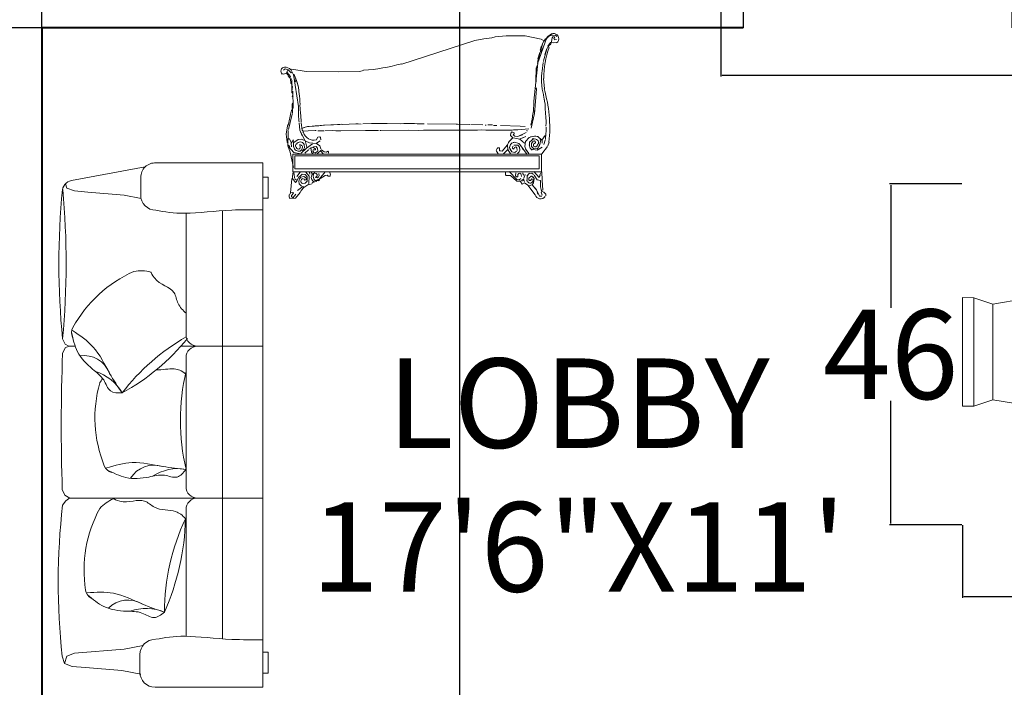
# Model space of a CAD drawing. Units: inches. Extents: x -124 to 612, y -69 to 524.
# Tile 4 of 9: x 16 to 148, y 240 to 329. Entities that reach past the tile are written whole.
import ezdxf
from ezdxf.enums import TextEntityAlignment as Align

# ---------------------------------------------------------------- set-up
doc = ezdxf.new("R2010")
doc.units = ezdxf.units.IN
doc.header["$MEASUREMENT"] = 0
for name, color, linetype, lineweight in [('A-ANNO-DIMS', 2, 'Continuous', 18), ('A-AREA-IDEN', 1, 'Continuous', 18), ('A-DOOR', 4, 'Continuous', 25), ('A-FURN', 8, 'Continuous', 18), ('A-WALL', 7, 'Continuous', 40)]:
    doc.layers.add(name, color=color, linetype=linetype, lineweight=lineweight)
doc.styles.get("Standard").update_dxf_attribs({"font": 'arial.ttf'})
doc.dimstyles.get("Standard").update_dxf_attribs({"dimtxt": 12, "dimasz": 0.18, "dimexe": 0.18, "dimexo": 0.0625, "dimgap": 0.09, "dimtad": 0, "dimtih": 1, "dimtoh": 1, "dimdec": 0, "dimzin": 0, "dimdsep": 46, "dimlunit": 4, "dimtxsty": 'Standard', "dimcen": 0.09, "dimadec": 0, "dimazin": 0, "dimtfac": 1, "dimtdec": 0, "dimtofl": 0, "dimtmove": 0, "dimatfit": 3, "dimfxl": 1, "dimtolj": 1, "dimtzin": 0, "dimarcsym": 0})

# ---------------------------------------------------------------- blocks, each defined once
blk = doc.blocks.new('A$C32C86113')
for p, q in [((82, 773.3, -9.2), (93.6, 803.8, -9.2)), ((93.6, 803.8, -9.2), (123, 812.9, -9.2)), ((736.9, 798.3, -9.2), (719.4, 811.4, -9.2)), ((747.8, 782.5, -9.2), (736.9, 798.3, -9.2)), ((747.6, 163.7, -9.2), (747.6, 782.8, -9.2)), ((747.7, 782.8, -9.2), (758.8, 802, -9.2)), ((758.8, 802, -9.2), (780.7, 812.4, -9.2)), ((1340.4, 800.9, -9.2), (1318.5, 811.4, -9.2)), ((1347.6, 787, -9.2), (1340.4, 800.9, -9.2)), ((1347.6, 787, -9.2), (1354.9, 800.9, -9.2)), ((1347.6, 787, -9.2), (1347.6, 761.5, -9.2)), ((1354.9, 800.9, -9.2), (1376.9, 811.5, -9.2)), ((77.9, 721.3, -9.2), (82, 773.3, -9.2)), ((2056, 484.9, -9.2), (2002, 776.1, -9.2)), ((65.8, 577.5, -9.2), (77.9, 721.3, -9.2)), ((51.2, 502.4, -9.2), (65.8, 577.5, -9.2)), ((60.2, 506.2, -9.2), (128.9, 506.2, -9.2)), ((2013.7, 502.6, -9.2), (1944.9, 502.8, -9.2)), ((0.2, 446.2, -9.2), (0, 20, -9.2)), ((2071.8, 20, 333.6), (2071.8, 442.4, 333.6)), ((702.6, 323.7, -9.2), (200, 323.4, -0.7)), ((1302.6, 323.7, -9.2), (792.6, 323.7, -9.2)), ((1347.6, 343.7, -9.2), (1347.6, 278.7, -9.2)), ((1872.8, 323.7, -9.2), (1392.6, 323.7, -9.2)), ((747.6, 20, -9.2), (747.6, 278.7, -9.2)), ((1347.6, 278.7, -9.2), (1347.6, 20, -9.2)), ((2071.8, 20, 333.6), (0, 20, -9.2)), ((55.9, 20), (55.9, 0)), ((139, 0), (139, 20, 13.8)), ((1932.8, 0), (1932.8, 20, 13.8)), ((2015.9, 20), (2015.9, 0)), ((55.9, 0), (139, 0)), ((2015.9, 0), (1932.8, 0))]:
    blk.add_line(p, q)
at = {"ltscale": 3}
for p, q in [((123, 794.8, -9.2), (93.6, 803.8, -9.2)), ((134.6, 764.2, -9.2), (123, 794.8, -9.2)), ((1960.7, 764.2, -9.2), (1972.3, 794.8, -9.2)), ((1972.3, 794.8, -9.2), (1989.3, 800, -9.2)), ((150.8, 568.4, -9.2), (134.6, 764.2, -9.2)), ((1956.6, 712.2, -9.2), (1960.7, 764.2, -9.2)), ((1944.5, 568.4, -9.2), (1956.6, 712.2, -9.2)), ((165.4, 493.4, -9.2), (150.8, 568.4, -9.2)), ((1931.4, 501.4, -9.2), (1944.5, 568.4, -9.2)), ((191.4, 179.1, 242), (1883, 179.1, 242))]:
    blk.add_line(p, q, dxfattribs=at)
for centre, radius, start, end in [((414.4, -1890.5, -9.2), 2719, 83.5605, 96.1533), ((1675, -2302.2, -9.2), 3127.9, 84.6632, 95.4698), ((1957.7, 767.9, -9.2), 45, 10.5091, 90), ((1399.9, 730.9, 333.6), 45, 61.3924, 113.2188), ((1178.3, 324.5, 333.6), 507.8, 23.7986, 61.3924), ((390.8, 676.1, 333.6), 45, 98.9106, 150.7371), ((462.5, 218.9, 333.6), 507.8, 61.3169, 98.9106), ((594.5, 543.8, 333.6), 164.4, 23.6986, 47.1794), ((1065.4, 175.7, 333.6), 507.8, 74.3829, 111.9767), ((1120.5, 522.1, 333.6), 164.4, 52.7695, 60.2454), ((892.1, 605, 333.6), 45, 111.9767, 163.8031), ((1917, 985.8, 333.6), 858.1, 208.4934, 231.1155), ((60.2, 446.2, -9.2), 60, 90, 179.9816), ((128.9, 446.2, -9.2), 60, 0, 90), ((1480.8, 501.9, 333.6), 164.4, 346.1804, 9.6612), ((1944.7, 442.8, -9.2), 60, 89.7859, 179.7859), ((2014.6, 445.3, 333.6), 57.3, 357.0581, 90.9206), ((691.5, 1297, 333.6), 971.5, 246.0331, 268.4688), ((702.6, 278.7, -9.2), 45, 0, 90), ((792.6, 278.7, -9.2), 45, 90, 180), ((1054.6, -512.3, 333.6), 858.1, 76.9593, 103.0407), ((1302.6, 278.7, -9.2), 45, 0, 90), ((1392.6, 278.7, -9.2), 45, 90, 180)]:
    blk.add_arc(centre, radius, start, end)
for centre, radius, start, end in [((1034.7, -7187.9, -9.2), 8004.3, 87.96784, 91.81809), ((1675, 3925.1, -9.2), 3127.9, 264.5302, 275.3368), ((1202.4, 727.4, 333.6), 108.4, 291.4614, 8.0497), ((1072.8, 736, 333.6), 183.2, 299.4203, 342.7126), ((236.2, 553.1, 333.6), 108.4, 328.9796, 45.568), ((639.9, -104, 333.6), 858.1, 29.8342, 52.4564), ((128.3, 481, 333.6), 183.2, 336.9386, 20.2309), ((769.4, 450.2, 333.6), 108.4, 342.0456, 58.634), ((680.5, 355.5, 333.6), 183.2, 350.0046, 33.2969), ((296.4, -448.9, 333.6), 858.1, 64.5272, 89.9746)]:
    blk.add_arc(centre, radius, start, end, dxfattribs=at)
for points, knots in [([(1402, 775.8, 333.6), (1375.6, 770, 333.6), (1319.1, 757.7, 333.6), (1261.1, 701.8, 333.6), (1222.2, 646.1, 333.6), (1162.2, 629.7, 333.6), (1162.6, 593.5, 333.6), (1162.8, 576.4, 333.6)], [0, 0, 0, 0, 79.746539, 170.719486, 232.023986, 283.143815, 329.425672, 329.425672, 329.425672, 329.425672]), ([(365.1, 713.1, 333.6), (347.7, 692.4, 333.6), (310.4, 648.2, 333.6), (298.4, 568.5, 333.6), (301.5, 500.7, 333.6), (263.9, 451.1, 333.6), (286.2, 422.7, 333.6), (296.8, 409.2, 333.6)], [0, 0, 0, 0, 79.746539, 170.719486, 232.023986, 283.143815, 329.425672, 329.425672, 329.425672, 329.425672]), ([(858.8, 635.1, 333.6), (846.5, 611.1, 333.6), (820.1, 559.5, 333.6), (826.5, 479.3, 333.6), (844.8, 413.9, 333.6), (819.4, 357.1, 333.6), (847.6, 334.4, 333.6), (860.9, 323.7, 333.6)], [0, 0, 0, 0, 79.746539, 170.719486, 232.023986, 283.143815, 329.425672, 329.425672, 329.425672, 329.425672]), ([(745, 609.9, 333.6), (745, 609.9, 333.6), (718.2, 560.7, 333.6), (755.5, 498.7, 333.6), (695.1, 438.3, 333.6), (705.8, 371.4, 333.6), (679.8, 337.8, 333.6), (665.5, 325.8, 333.6)], [27.786417, 27.786417, 27.786417, 27.786417, 60.334214, 153.42843, 198.910048, 289.238615, 341.466319, 341.466319, 341.466319, 341.466319]), ([(189.7, 443.1, -9.2), (195.9, 408.3, 46.7), (209, 335.3, 164.5), (187, 169.8, 251), (187.5, 61.2, 288.7), (187.7, 20, 303)], [0, 0, 0, 0, 194.838243, 409.817627, 541.189597, 541.189597, 541.189597, 541.189597]), ([(1253.9, 441, 333.6), (1252.3, 416.7, 333.6), (1266, 375.1, 333.6), (1250.1, 340.7, 333.6), (1238.9, 325.8, 333.6)], [214.332348, 214.332348, 214.332348, 214.332348, 289.238615, 341.466319, 341.466319, 341.466319, 341.466319]), ([(1640.5, 462.6, 333.6), (1640.5, 462.6, 333.6), (1589.2, 439.9, 333.6), (1581.1, 368, 333.6), (1510.9, 358.8, 333.6), (1488.8, 335.7, 333.6), (1477.6, 323.7, 333.6)], [27.786417, 27.786417, 27.786417, 27.786417, 60.334214, 153.42843, 198.910048, 250.027656, 250.027656, 250.027656, 250.027656]), ([(1884.7, 443.1, -9.2), (1878.5, 408.3, 46.7), (1865.4, 335.3, 164.5), (1887.4, 169.8, 251), (1886.9, 61.2, 288.7), (1886.7, 20, 303)], [0, 0, 0, 0, 194.838243, 409.817627, 541.189597, 541.189597, 541.189597, 541.189597])]:
    blk.add_open_spline(points, degree=3, knots=knots)
for points in [[(1409.2, 771.8, 333.6), (1389.5, 742.5, 333.6), (1346.6, 678.6, 333.6), (1247.3, 632.8, 333.6), (1188.1, 593.3, 333.6), (1162.8, 576.4, 333.6)], [(373.3, 714.3, 333.6), (375.5, 679, 333.6), (380.4, 602.2, 333.6), (329.5, 505.4, 333.6), (306.6, 438, 333.6), (296.8, 409.2, 333.6)], [(866.4, 638.2, 333.6), (876.6, 604.3, 333.6), (898.7, 530.5, 333.6), (871, 424.8, 333.6), (864, 353.9, 333.6), (860.9, 323.7, 333.6)]]:
    blk.add_open_spline(points, degree=3, knots=[0, 0, 0, 0, 104.254828, 226.968516, 318.497377, 318.497377, 318.497377, 318.497377], dxfattribs=at)
blk = doc.blocks.new('A$C0D2616A3')
for p, q in [((673.1, 750.4), (1080.1, 881.7)), ((1080.1, 881.7), (1130.6, 891.6)), ((1130.6, 891.6), (1175.6, 896.2)), ((1175.6, 896.2), (1193.7, 901.3)), ((1193.7, 901.3), (1254.9, 907.4)), ((1254.9, 907.4), (1361, 907.4)), ((1361, 907.4), (1450.6, 889.6)), ((1430.2, 751.5), (1481.4, 898.1)), ((1450.6, 889.6), (1463.1, 882.2)), ((1474, 891), (1463, 875)), ((1483.1, 892.7), (1474, 891)), ((1479.4, 889.1), (1474, 891)), ((1477.7, 892.8), (1479.4, 889.1)), ((1481.4, 898.1), (1490.5, 906.9)), ((1483.1, 896.3), (1481.4, 898.1)), ((1494.1, 905.1), (1483.1, 896.3)), ((1503.1, 910.3), (1490.5, 906.9)), ((1497.7, 908.6), (1512.2, 913.7)), ((1530.1, 911.6), (1503.1, 910.3)), ((1506, 865.3), (1510.1, 895.8)), ((1510.1, 895.8), (1515.6, 902.9)), ((1515.6, 902.9), (1522.8, 902.8)), ((1526.3, 897.3), (1520.8, 892)), ((1520.8, 892), (1524.3, 884.8)), ((1522.8, 902.8), (1526.3, 897.3)), ((1524.3, 884.8), (1535.1, 886.4)), ((1537.2, 904.3), (1530.1, 911.6)), ((1428.6, 760.5), (1459.2, 867.9)), ((1444.2, 828.6), (1451.8, 851.9)), ((1449.4, 817.7), (1460.6, 844.5)), ((1455.5, 859), (1463, 875)), ((1466.7, 781.5), (1480.1, 828)), ((1470.7, 803), (1482.1, 836.9)), ((1482, 833.3), (1487.6, 844)), ((1487.7, 849.4), (1502.5, 870.7)), ((1493, 843.9), (1487.7, 849.4)), ((1491.3, 851.2), (1504.1, 861.7)), ((1502.5, 870.7), (1507.9, 872.5)), ((1507.9, 872.5), (1516.8, 868.7)), ((1516.8, 868.7), (1534.8, 870.2)), ((1430.7, 780.3), (1442.1, 814.3)), ((1462.9, 765.3), (1464.8, 776.1)), ((1464.8, 776.1), (1466.7, 781.5)), ((23.5, 723.9), (14.4, 716.9)), ((39.6, 718.3), (23.5, 723.9)), ((33.9, 704), (35.9, 714.7)), ((57.3, 701.8), (39.6, 718.3)), ((67.9, 694.4), (55.8, 719.8)), ((57.6, 719.7), (61.2, 721.5)), ((61.2, 721.5), (140.1, 709.3)), ((438.7, 709.5), (460.3, 714.5)), ((1408.6, 543.3), (1430.3, 755.1)), ((1419.6, 656.4), (1422.6, 726.5)), ((1422.6, 726.5), (1428.3, 742.6)), ((1454.7, 711.5), (1460.9, 758.2)), ((8.6, 695.4), (15.8, 693.5)), ((15.8, 693.5), (28.5, 698.7)), ((30.3, 700.4), (33.9, 704)), ((37.3, 691.3), (30.3, 700.4)), ((41, 698.4), (35.7, 703.9)), ((44.5, 691.2), (37.3, 691.3)), ((40.8, 684.1), (41, 698.4)), ((47.8, 675), (40.8, 684.1)), ((53.3, 680.2), (44.5, 691.2)), ((47.8, 671.4), (53.3, 680.2)), ((53.1, 667.7), (54.5, 644.3)), ((60.2, 660.3), (55, 671.2)), ((62.7, 703.5), (57.3, 701.8)), ((60.8, 592), (60.2, 660.3)), ((97.2, 514), (69.7, 692.6)), ((69.7, 692.6), (73.3, 692.5)), ((73.3, 692.5), (92.2, 641.8)), ((81.6, 651), (78.2, 663.6)), ((83.7, 670.7), (78.5, 681.6)), ((97.3, 621.9), (85.4, 663.5)), ((140.1, 709.3), (323.5, 706.1)), ((323.5, 706.1), (438.7, 709.5)), ((1422.2, 704.9), (1427.7, 710.2)), ((1451.8, 645), (1452.3, 673.8)), ((1452.3, 673.8), (1452.4, 679.2)), ((1452.4, 679.2), (1452.8, 702.6)), ((1452.8, 702.6), (1454.7, 711.5)), ((1469.2, 612.4), (1463, 670)), ((54.5, 644.3), (63.3, 636.9)), ((60.8, 595.6), (65, 626.1)), ((63.2, 629.7), (61.4, 628)), ((65, 626.1), (63.2, 629.7)), ((95.5, 627.4), (93.9, 636.4)), ((101.9, 580.5), (97.3, 621.9)), ((1412.8, 473.1), (1424.2, 611.4)), ((1423.1, 652.7), (1419.6, 656.4)), ((1424.2, 611.4), (1420.7, 618.6)), ((1453.4, 636), (1451.8, 645)), ((1453.2, 623.4), (1453.4, 636)), ((1454.9, 618), (1453.2, 623.4)), ((1454.8, 610.8), (1454.9, 618)), ((1463.2, 580.1), (1454.8, 610.8)), ((66.1, 586.5), (60.8, 592)), ((62.2, 570.4), (65.9, 575.7)), ((67.5, 564.9), (62.2, 570.4)), ((68.2, 505.6), (66.3, 599.1)), ((103.6, 575.1), (101.9, 580.5)), ((103.5, 567.9), (103.6, 575.1)), ((105.2, 560.7), (103.5, 567.9)), ((104.8, 537.3), (105.2, 560.7)), ((1464.7, 563.9), (1463.2, 578.3)), ((1468.1, 549.5), (1464.7, 563.9)), ((1468, 544.1), (1466.4, 554.9)), ((55.2, 478.8), (60.9, 496.7)), ((63.2, 527.2), (66.9, 532.6)), ((64.1, 475.1), (63.2, 527.2)), ((64.6, 502), (68.2, 505.6)), ((98.9, 508.6), (97.2, 514)), ((98.1, 467.3), (98.8, 503.2)), ((98.8, 503.2), (98.9, 508.6)), ((106.4, 530.1), (104.8, 537.3)), ((106.2, 515.7), (106.4, 530.1)), ((107.9, 508.5), (106.2, 515.7)), ((107.6, 494.1), (107.9, 508.5)), ((109.2, 481.5), (107.6, 494.1)), ((1408.4, 532.5), (1407.7, 491.2)), ((1408.5, 537.9), (1408.4, 532.5)), ((1408.5, 537.9), (1408.6, 543.3)), ((1471.3, 526), (1468, 544.1)), ((1471.1, 518.8), (1471.3, 526)), ((1472.7, 504.4), (1471.1, 518.8)), ((1472.5, 493.6), (1472.7, 504.4)), ((1474.2, 486.4), (1472.5, 493.6)), ((41.5, 416.1), (55.2, 478.8)), ((42.8, 385.5), (62.3, 471.5)), ((99.3, 433.1), (98.1, 467.3)), ((112, 434.7), (109.2, 481.5)), ((1393.4, 392.5), (1410.9, 467.7)), ((1397.8, 435.6), (1399.6, 441)), ((1399.6, 441), (1401.8, 458.9)), ((1401.8, 458.9), (1403.8, 475)), ((1405.8, 482.2), (1403.7, 469.7)), ((1411.2, 487.5), (1405.8, 482.2)), ((1407.7, 491.2), (1411.2, 487.5)), ((1410.9, 467.7), (1412.8, 473.1)), ((1473.9, 468.4), (1474.2, 486.4)), ((1475.5, 461.2), (1473.9, 468.4)), ((1475.3, 450.4), (1475.5, 461.2)), ((1476.9, 434.2), (1475.3, 450.4)), ((29.7, 358.8), (35.9, 405.4)), ((35.9, 405.4), (41.5, 416.1)), ((101.1, 427.7), (99.3, 433.1)), ((105.7, 382.6), (101, 422.3)), ((113.6, 427.4), (112, 434.7)), ((113.5, 422), (118.2, 382.4)), ((118.4, 391.4), (134.7, 398.3)), ((123.9, 394.9), (147.4, 401.7)), ((158.1, 401.5), (147.4, 401.7)), ((158.1, 401.5), (174.4, 404.8)), ((185.2, 404.6), (174.4, 404.8)), ((185.2, 404.6), (190.6, 406.3)), ((212.2, 405.9), (190.6, 406.3)), ((212.2, 405.9), (219.4, 407.6)), ((226.6, 407.5), (219.4, 407.6)), ((226.6, 407.5), (237.4, 409.1)), ((242.8, 409), (237.4, 409.1)), ((242.8, 409), (278.8, 412)), ((293.2, 411.7), (278.8, 412)), ((293.2, 411.7), (314.8, 413.1)), ((327.4, 412.9), (314.8, 413.1)), ((327.4, 412.9), (336.4, 414.6)), ((343.6, 414.4), (336.4, 414.6)), ((343.6, 414.4), (417.4, 416.7)), ((429.9, 416.5), (417.4, 416.7)), ((447.9, 416.2), (429.9, 416.5)), ((456.9, 417.8), (505.5, 418.8)), ((510.9, 418.7), (505.5, 418.8)), ((510.9, 418.7), (584.6, 419.2)), ((591.8, 419.1), (584.6, 419.2)), ((665.5, 417.8), (591.8, 419.1)), ((665.5, 417.8), (685.3, 419.3)), ((744.7, 418.2), (685.3, 419.3)), ((759.1, 418), (744.7, 418.2)), ((771.6, 417.7), (759.1, 418)), ((798.6, 417.3), (771.6, 417.7)), ((816.6, 417), (976.6, 416)), ((983.8, 415.8), (976.6, 416)), ((1052.1, 412.9), (983.8, 415.8)), ((1124, 411.6), (1057.5, 412.8)), ((1143.7, 409.5), (1138.3, 409.6)), ((1177.9, 410.7), (1152.8, 411.1)), ((1203.1, 408.4), (1185.1, 408.7)), ((1332.5, 404.4), (1222.8, 408.1)), ((1380.8, 389.1), (1319.5, 383)), ((1361.2, 402.1), (1332.5, 404.4)), ((1391.9, 410.5), (1397.8, 435.6)), ((1476.3, 403.7), (1476.7, 423.4)), ((1476.7, 423.4), (1476.9, 434.2)), ((1477.6, 373.1), (1477.8, 387.4)), ((1477.8, 387.4), (1477.9, 392.8)), ((1477.9, 392.8), (1478, 398.2)), ((34.4, 315.5), (29.7, 358.8)), ((39.4, 293.9), (40.9, 380.2)), ((41.8, 331.6), (45.5, 335.1)), ((45.5, 335.1), (54.3, 322.4)), ((95.8, 330.6), (72.1, 313.1)), ((115.6, 332.1), (95.8, 330.6)), ((117.7, 350), (105.7, 382.6)), ((131.7, 328.2), (107.4, 379)), ((160.2, 311.5), (115.6, 332.1)), ((118.2, 382.4), (123.5, 376.9)), ((123.5, 376.9), (123.4, 367.9)), ((125.3, 376.9), (152.3, 378.2)), ((135.6, 347.9), (126.9, 360.7)), ((152.3, 378.2), (190.1, 379.3)), ((197.3, 379.2), (190.1, 379.3)), ((196.4, 327.1), (205.7, 343.1)), ((205.7, 343.1), (216.5, 344.7)), ((238.7, 378.5), (206.3, 379.1)), ((216.5, 344.7), (220, 341.1)), ((220, 341.1), (221.6, 328.4)), ((244.1, 378.4), (285.4, 379.5)), ((305.2, 379.1), (285.4, 379.5)), ((310.6, 379), (305.2, 379.1)), ((319.6, 378.9), (310.6, 379)), ((325, 378.8), (319.6, 378.9)), ((334, 378.6), (325, 378.8)), ((334, 378.6), (470.7, 379.8)), ((494, 379.4), (470.7, 379.8)), ((494, 379.4), (544.4, 380.4)), ((557, 380.1), (551.6, 380.2)), ((557, 380.1), (708.1, 381.1)), ((769.2, 380), (708.1, 381.1)), ((769.2, 380), (794.4, 381.4)), ((801.6, 381.3), (794.4, 381.4)), ((801.6, 381.3), (905.9, 381.2)), ((916.7, 381.1), (900.5, 381.3)), ((916.7, 381.1), (976, 381.8)), ((1008.4, 381.2), (976, 381.8)), ((1008.4, 381.2), (1044.4, 382.4)), ((1094.7, 381.5), (1044.4, 382.4)), ((1094.7, 381.5), (1118.1, 382.9)), ((1141.5, 382.5), (1118.1, 382.9)), ((1146.9, 382.4), (1141.5, 382.5)), ((1157.6, 382.2), (1146.9, 382.4)), ((1157.6, 382.2), (1236.8, 382.7)), ((1269.1, 382.1), (1236.8, 382.7)), ((1281.7, 381.9), (1269.1, 382.1)), ((1271.6, 319.1), (1288.1, 335)), ((1281.4, 365.7), (1279.4, 353.1)), ((1279.4, 353.1), (1291.8, 338.5)), ((1287, 372.8), (1281.4, 365.7)), ((1288.9, 381.7), (1281.7, 381.9)), ((1291.8, 338.5), (1282.6, 331.5)), ((1288.9, 381.7), (1296.1, 383.4)), ((1293.6, 338.5), (1331.2, 332.5)), ((1302.7, 349.1), (1293.9, 356.5)), ((1319.5, 383), (1296.1, 383.4)), ((1318.9, 347.1), (1302.7, 349.1)), ((1366, 369.6), (1318.9, 347.1)), ((1329.7, 350.5), (1346, 355.6)), ((1331.2, 332.5), (1356, 308.6)), ((1333, 334.2), (1363.8, 346.3)), ((1342.1, 337.7), (1352.9, 341.1)), ((1383.5, 340.5), (1361.6, 319.3)), ((1371.5, 376.7), (1369.8, 382.1)), ((1399.8, 347.4), (1383.5, 340.5)), ((1384.9, 315.3), (1408.6, 334.7)), ((1390.8, 344), (1407, 347.3)), ((1399.6, 333.1), (1406.8, 334.7)), ((1407, 347.3), (1412.4, 349)), ((1419.6, 348.9), (1412.4, 349)), ((1426.8, 347), (1419.6, 348.9)), ((1426.8, 347), (1430.4, 346.9)), ((1430.4, 346.9), (1453.4, 326.7)), ((1444.4, 328.7), (1448.1, 334)), ((1453.4, 326.7), (1471.8, 351.6)), ((1458.9, 332), (1466.4, 348.1)), ((1473.2, 330), (1475.7, 365.9)), ((1475.7, 365.9), (1477.6, 373.1)), ((39.7, 310), (34.4, 315.5)), ((51.4, 259.5), (39.4, 293.9)), ((71.1, 257.3), (42.9, 290.2)), ((50.1, 288.3), (43.1, 299.2)), ((46.4, 284.7), (48.3, 291.9)), ((54.3, 322.4), (55.9, 315.2)), ((57.6, 309.7), (70.5, 327.5)), ((59.1, 288.1), (57.6, 309.7)), ((68.6, 322.1), (70.3, 313.1)), ((70.3, 313.1), (69.8, 287.9)), ((80.8, 296.7), (84.5, 305.7)), ((82.4, 287.7), (80.8, 296.7)), ((104.2, 299.9), (107.7, 292.7)), ((107.2, 265.7), (116.4, 274.5)), ((112.4, 253), (143.5, 281.3)), ((129, 277.9), (119.9, 269.1)), ((129.4, 303.1), (130.9, 281.5)), ((145.3, 286.6), (135.2, 324.6)), ((143.5, 281.3), (176.3, 305.9)), ((177.7, 287.9), (155.9, 275.6)), ((197.9, 307.3), (160.2, 311.5)), ((166.9, 284.4), (170, 259.2)), ((192, 278.6), (177.7, 287.9)), ((195.8, 291.1), (181.4, 289.6)), ((191.8, 271.4), (192, 278.6)), ((204.6, 282), (195.8, 291.1)), ((197.9, 309.1), (217.9, 323.1)), ((217.4, 294.4), (197.9, 307.3)), ((206.1, 265.8), (204.6, 282)), ((222.5, 278.1), (217.4, 294.4)), ((1200.7, 271.8), (1204.4, 278.9)), ((1204.4, 278.9), (1208.1, 284.3)), ((1208.1, 284.3), (1217.1, 284.1)), ((1217.1, 284.1), (1216.8, 266.1)), ((1218.6, 266.1), (1217, 278.7)), ((1232.9, 265.8), (1262.3, 299.5)), ((1239.9, 249.5), (1263.7, 274.3)), ((1263.7, 276.1), (1262.2, 295.9)), ((1262.3, 299.5), (1266.1, 308.4)), ((1263.7, 274.3), (1279.4, 250.6)), ((1266.1, 308.4), (1267.9, 313.8)), ((1267.9, 313.8), (1271.6, 319.1)), ((1272.8, 284.9), (1278.5, 302.8)), ((1279.7, 268.6), (1272.8, 284.9)), ((1286.8, 261.3), (1274.5, 279.5)), ((1278.5, 302.8), (1287.7, 311.6)), ((1290.8, 281), (1292.8, 293.6)), ((1294.3, 277.4), (1290.8, 281)), ((1296.7, 313.3), (1291.3, 313.4)), ((1297.8, 275.5), (1294.3, 277.4)), ((1296.7, 313.3), (1302.1, 315)), ((1301.6, 286.2), (1297.8, 275.5)), ((1319.8, 298.5), (1298.3, 298.9)), ((1308.9, 289.7), (1301.6, 286.2)), ((1325.4, 307.4), (1302.1, 315)), ((1314.2, 284.2), (1308.9, 289.7)), ((1315.7, 268), (1314.2, 284.2)), ((1328.6, 287.5), (1319.8, 298.5)), ((1330.7, 301.9), (1325.4, 307.4)), ((1330.1, 271.3), (1328.6, 287.5)), ((1371.1, 247.2), (1330.7, 301.9)), ((1350, 272.8), (1337.7, 292.8)), ((1359.3, 290.6), (1361.6, 319.3)), ((1367.8, 265.3), (1359.3, 290.6)), ((1380.2, 252.5), (1362.6, 278)), ((1387.9, 281.1), (1382.8, 301)), ((1384.5, 295.6), (1384.9, 315.3)), ((1400.3, 270.1), (1387.9, 281.1)), ((1427.2, 269.6), (1393.2, 275.6)), ((1395.5, 308), (1395.2, 290)), ((1395.2, 290), (1407.6, 279)), ((1404.7, 320.4), (1395.5, 308)), ((1412, 322.1), (1404.7, 320.4)), ((1406.2, 304.2), (1419, 311.1)), ((1407.9, 293.4), (1406.2, 304.2)), ((1407.6, 279), (1427.4, 278.6)), ((1415, 289.6), (1407.9, 293.4)), ((1419, 314.7), (1412, 322.1)), ((1420.4, 289.5), (1415, 289.6)), ((1419, 311.1), (1419, 314.7)), ((1427.7, 294.8), (1420.4, 289.5)), ((1425.8, 293), (1431.4, 305.5)), ((1454.5, 287.1), (1427.2, 269.6)), ((1427.4, 278.6), (1432.9, 283.9)), ((1429.6, 300.2), (1427.7, 294.8)), ((1432.9, 283.9), (1444.1, 308.9)), ((1438.4, 291), (1442.2, 301.7)), ((1444.1, 308.9), (1446.1, 323.3)), ((1446.1, 323.3), (1444.4, 328.7)), ((1453.8, 249.4), (1485.1, 290.2)), ((1454.9, 308.7), (1455.2, 324.9)), ((1465.5, 301.3), (1471.4, 326.4)), ((1487, 293.8), (1494.6, 315.2)), ((69.7, 174.6), (51.4, 259.5)), ((67.3, 247.8), (1452.3, 247.8)), ((67.3, 149.6), (67.3, 247.8)), ((110.5, 249.5), (71.1, 257.3)), ((78.4, 239.6), (1438.7, 239.6)), ((78.4, 165.9), (78.4, 239.6)), ((119.9, 269.1), (114.5, 271)), ((154.1, 272.1), (134, 254.4)), ((170, 259.2), (177.1, 250.1)), ((177.3, 264.5), (179.3, 271.6)), ((186.2, 255.3), (177.3, 264.5)), ((179.3, 271.6), (191.8, 271.4)), ((189.7, 253.5), (204.3, 262.2)), ((202.2, 249.7), (226, 272.6)), ((238.2, 249), (222.3, 265.5)), ((226, 272.6), (240.2, 261.6)), ((240.2, 261.6), (254.6, 259.5)), ((254.6, 259.5), (261.9, 264.8)), ((261.9, 264.8), (265.4, 261.1)), ((265.4, 261.1), (265.3, 254)), ((1198.8, 268.2), (1211.1, 250)), ((1216.8, 266.1), (1232.9, 265.8)), ((1302.9, 257.4), (1286.8, 261.3)), ((1312, 264.5), (1302.9, 257.4)), ((1317.2, 251.8), (1326.4, 260.6)), ((1326.4, 260.6), (1330.1, 271.3)), ((1438.7, 239.6), (1438.7, 165.9)), ((1452.3, 247.8), (1452.3, 149.6)), ((1438.7, 165.9), (78.4, 165.9)), ((52.8, 32.9), (61.3, 110.1)), ((61.3, 110.1), (65.1, 119)), ((80.8, 89.9), (65, 111.8)), ((65.1, 119), (67.3, 144.1)), ((1452.3, 149.6), (67.3, 149.6)), ((74.4, 136.8), (71, 149.4)), ((75.8, 115.2), (74.4, 136.8)), ((86.4, 104.2), (77.6, 111.6)), ((99.3, 120.2), (86.3, 95.2)), ((88.6, 124), (106.9, 147)), ((99.3, 120.2), (108.4, 127.2)), ((102.6, 103.9), (104.5, 111.1)), ((104.5, 111.1), (111.9, 120)), ((119.3, 136), (108.4, 127.2)), ((111.9, 120), (128.1, 123.3)), ((135.5, 135.7), (119.3, 136)), ((128.1, 123.3), (137, 117.7)), ((146.1, 121.2), (135.5, 135.7)), ((156.9, 126.4), (137.6, 150.1)), ((145.6, 97.8), (146.1, 121.2)), ((156.2, 85), (156.9, 126.4)), ((160.7, 137.1), (159.1, 146.1)), ((173.4, 140.5), (166.3, 149.6)), ((196.7, 140.1), (186, 143.8)), ((246.9, 130.2), (192.4, 95.2)), ((192.8, 118.6), (201.9, 127.4)), ((203.5, 116.6), (192.8, 118.6)), ((202, 134.6), (196.7, 140.1)), ((201.9, 127.4), (202, 134.6)), ((210.8, 123.6), (203.5, 116.6)), ((211.1, 139.8), (212.7, 127.2)), ((214.2, 111), (247.3, 150)), ((257.7, 131.8), (246.9, 130.2)), ((263, 126.3), (257.7, 131.8)), ((272, 126.2), (263, 126.3)), ((275.7, 129.7), (272, 126.2)), ((275.7, 133.3), (272.4, 145.9)), ((1250.4, 132.5), (1250.7, 150.4)), ((1253.9, 128.8), (1250.4, 132.5)), ((1279.1, 130.2), (1253.9, 128.8)), ((1314.7, 106.2), (1272.3, 151.9)), ((1314.5, 97.2), (1279.1, 130.2)), ((1308.1, 144), (1306.1, 127.9)), ((1306.1, 127.9), (1313.2, 122.4)), ((1313.2, 122.4), (1320.4, 122.2)), ((1320.4, 122.2), (1320.6, 136.6)), ((1336.4, 113), (1327.3, 105.9)), ((1340.2, 123.7), (1338.5, 134.5)), ((1350.7, 110.9), (1346.9, 98.4)), ((1347.7, 143.3), (1347.6, 138)), ((1347.6, 138), (1352.9, 130.7)), ((1357.7, 96.4), (1350.7, 110.9)), ((1352.6, 114.5), (1360.1, 134.1)), ((1369, 125), (1385.4, 142.7)), ((1372.7, 133.9), (1370.3, 98)), ((1381.2, 105), (1381.3, 114)), ((1381.3, 114), (1394.2, 126.4)), ((1398, 142.5), (1381.8, 141)), ((1397.5, 110.1), (1390.1, 101.2)), ((1394.2, 126.4), (1397.7, 126.3)), ((1404.6, 106.4), (1397.5, 110.1)), ((1406.6, 117.1), (1397.7, 126.3)), ((1406.9, 135.1), (1398, 142.5)), ((1403.1, 122.6), (1410.1, 113.5)), ((1410.1, 113.5), (1407.9, 88.3)), ((1409, 151.3), (1439, 118.4)), ((1428, 106), (1410.4, 131.5)), ((1439, 118.4), (1444.7, 136.3)), ((1440.8, 120.1), (1444.6, 129.1)), ((1444.7, 136.3), (1448.4, 143.4)), ((1454.9, 103.7), (1453.9, 150.5)), ((86.3, 95.2), (80.8, 89.9)), ((92.6, 44.8), (121.7, 67.6)), ((100.7, 98.6), (102.6, 103.9)), ((102.2, 82.4), (100.7, 98.6)), ((114.6, 69.6), (102.2, 82.4)), ((112.4, 46.2), (127, 62.2)), ((120.3, 85.6), (134.7, 87.2)), ((121.7, 67.6), (125.3, 64)), ((127, 62.2), (156.2, 81.4)), ((134.7, 87.2), (145.6, 97.8)), ((156.2, 81.4), (159.7, 79.6)), ((159.7, 79.6), (172.4, 82.9)), ((181.5, 93.6), (174.2, 86.5)), ((188.7, 93.4), (181.5, 93.6)), ((201.5, 105.8), (194.2, 100.5)), ((210.4, 100.3), (201.5, 105.8)), ((217.7, 103.7), (207, 107.5)), ((210.6, 109.2), (210.4, 100.3)), ((1337.9, 98.6), (1314.5, 97.2)), ((1327.3, 105.9), (1314.7, 106.2)), ((1344.8, 80.5), (1334.3, 95)), ((1339.8, 102.1), (1347.1, 107.4)), ((1357.5, 89.2), (1344.8, 80.5)), ((1375.3, 76.3), (1357.5, 89.2)), ((1415.7, 21.7), (1375.3, 76.3)), ((1384.7, 101.3), (1381.2, 105)), ((1382.4, 72.6), (1396.9, 77.8)), ((1390.1, 101.2), (1384.7, 101.3)), ((1407.9, 88.3), (1398.7, 77.7)), ((1398.7, 77.7), (1419.9, 54)), ((1423.4, 48.5), (1416.4, 59.4)), ((1445.9, 102.1), (1428, 106)), ((1445.3, 66.1), (1445.4, 76.9)), ((1452.1, 44.4), (1445.3, 66.1)), ((1445.4, 76.9), (1445.6, 85.9)), ((1445.6, 85.9), (1445.9, 102.1)), ((1459.3, 47.9), (1454.9, 103.7)), ((81.1, 3.6), (50.4, 0.5)), ((67.2, 34.4), (54.6, 32.8)), ((59.6, 13), (59.7, 18.4)), ((70.3, 3.8), (59.6, 13)), ((59.7, 18.4), (70.7, 30.8)), ((70.7, 30.8), (67.2, 34.4)), ((68.5, 7.4), (83.2, 25.2)), ((106.8, 33.7), (81.1, 3.6)), ((108.6, 37.3), (112.4, 46.2)), ((1423.4, 48.5), (1440.7, 14)), ((1431.9, 25), (1426.8, 37.7)), ((1440.7, 14), (1453.3, 13.8)), ((1453.8, 39), (1450.1, 35.5)), ((1450.1, 35.5), (1455.2, 19.2)), ((1455.6, 40.8), (1450.3, 48)), ((1459.2, 42.5), (1455.6, 40.8)), ((1462.8, 38.8), (1475.1, 26)), ((1475.1, 26), (1474.9, 15.2))]:
    blk.add_line(p, q)
for centre, radius, start, end in [((1519, 892), 28.8, 305.8699, 146.9946), ((1914.6, 681.9), 449.5, 158.9779, 181.5094), ((21.5, 711.4), 21.6, 93.3987, 231.125), ((24.8, 693.3), 39.6, 40.4237, 96.4314), ((379, 1827.3), 1114.8, 274.1777, 285.275), ((746.1, 396.6), 751.6, 353.7932, 16.6146), ((183, 384.9), 59.3, 195.8584, 283.0362), ((1292.2, 363.7), 7.19, 283.0362, 119.9638), ((1413.6, 311.2), 21.6, 342.3008, 106.1027), ((100.5, 292.8), 28.8, 189.008, 283.9314), ((96.8, 287.5), 10.8, 179, 25.5651), ((107.7, 292.7), 23.4, 25.5651, 150.6992), ((107.6, 287.3), 12.6, 319.1944, 104.9454), ((125.9, 98.1), 14.4, 103.0362, 245.8014), ((135.1, 110.6), 7.19, 170.8699, 74.9638), ((196.4, 118.5), 27, 124.5377, 234.3048), ((210.9, 125.4), 30.6, 136.1211, 249.56), ((1329.5, 132.9), 8.99, 10.3099, 157.1986), ((1388.4, 103.1), 16.2, 195.6992, 11.5288), ((63.3, 14.7), 18, 119.9638, 227.8141), ((1446.5, 31.9), 32.4, 198.44, 322.7462)]:
    blk.add_arc(centre, radius, start, end)
blk = doc.blocks.new('A$C6C037A94')
for p, q in [((0.7877, 1.6959), (0.4032, 1.6959)), ((0.4032, 1.6959), (0.4039, 1.6557)), ((0.7877, 1.6557), (0.7877, 1.6959)), ((0.4258, 1.588), (0.4039, 1.6557)), ((0.7877, 1.6557), (0.4039, 1.6557)), ((0.7658, 1.588), (0.7877, 1.6557)), ((0.407, 1.4737), (0.4258, 1.588)), ((0.7658, 1.588), (0.4258, 1.588)), ((0.7847, 1.4737), (0.7658, 1.588)), ((0.307, 1.4737), (0.8868, 1.4737)), ((0.327, 1.4537), (0.8668, 1.4537)), ((0.227, 0.2974), (0.227, 1.3937)), ((0.247, 0.3174), (0.247, 1.3737)), ((0.9468, 1.3737), (0.9468, 0.3174)), ((0.9668, 1.3937), (0.9668, 0.2974)), ((0, 1.2552), (0, 0.8707)), ((0.0402, 1.2552), (0, 1.2552)), ((0.0402, 1.2552), (0.0402, 0.8714)), ((0.1079, 1.2333), (0.0402, 1.2552)), ((0.227, 1.2529), (0.1079, 1.2333)), ((0.1079, 1.2333), (0.1079, 0.8933)), ((0.9668, 1.2553), (1.1005, 1.2333)), ((1.1005, 1.2333), (1.1682, 1.2552)), ((1.1005, 1.2333), (1.1005, 0.8933)), ((1.1682, 1.2552), (1.2084, 1.2552)), ((1.1682, 1.2552), (1.1682, 0.8714)), ((1.2084, 1.2552), (1.2084, 0.8707)), ((0.1079, 0.8933), (0.0402, 0.8714)), ((0.227, 0.8736), (0.1079, 0.8933)), ((0.9668, 0.8712), (1.1005, 0.8933)), ((1.1005, 0.8933), (1.1682, 0.8714)), ((0, 0.8707), (0.0402, 0.8714)), ((1.2084, 0.8707), (1.1682, 0.8714)), ((0, 0.7888), (0, 0.4043)), ((0.0402, 0.7888), (0, 0.7888)), ((0.0402, 0.7888), (0.0402, 0.405)), ((0.1079, 0.7669), (0.0402, 0.7888)), ((0.227, 0.7865), (0.1079, 0.7669)), ((0.9668, 0.7889), (1.1005, 0.7669)), ((1.1005, 0.7669), (1.1682, 0.7888)), ((1.1682, 0.7888), (1.1682, 0.405)), ((1.1682, 0.7888), (1.2084, 0.7888)), ((1.2084, 0.7888), (1.2084, 0.4043)), ((0.1079, 0.7669), (0.1079, 0.4269)), ((1.1005, 0.7669), (1.1005, 0.4269)), ((0.1079, 0.4269), (0.0402, 0.405)), ((0.227, 0.4072), (0.1079, 0.4269)), ((0.9668, 0.4048), (1.1005, 0.4269)), ((1.1005, 0.4269), (1.1682, 0.405)), ((0, 0.4043), (0.0402, 0.405)), ((1.2084, 0.4043), (1.1682, 0.405)), ((0.8868, 0.2174), (0.307, 0.2174)), ((0.8668, 0.2374), (0.327, 0.2374)), ((0.4078, 0.2174), (0.4258, 0.1079)), ((0.7839, 0.2174), (0.7658, 0.1079)), ((0.4258, 0.1079), (0.4039, 0.0402)), ((0.7658, 0.1079), (0.4258, 0.1079)), ((0.7658, 0.1079), (0.7877, 0.0402)), ((0.4032, 0), (0.4039, 0.0402)), ((0.7877, 0.0402), (0.4039, 0.0402)), ((0.7877, 0.0402), (0.7877, 0)), ((0.7877, 0), (0.4032, 0))]:
    blk.add_line(p, q)
for centre, start, end in [((0.307, 1.3937), 90, 180), ((0.8868, 1.3937), 360, 90), ((0.327, 1.3737), 90, 180), ((0.8668, 1.3737), 360, 90), ((0.327, 0.3174), 180, 270), ((0.8668, 0.3174), 270, 0), ((0.307, 0.2974), 180, 270), ((0.8868, 0.2974), 270, 360)]:
    blk.add_arc(centre, 0.08, start, end)
blk = doc.blocks.new('DOOR-36IN-SINGLE')
for p, q in [((0, 6), (0, 0)), ((3, 6), (3, 0)), ((39, 6), (39, 0)), ((42, 6), (42, 0))]:
    blk.add_line(p, q)
blk.add_lwpolyline([(39, 6), (36, 6), (36, 42), (39, 42)], close=True)
blk.add_arc((37.5, 7.5), 34.53, 87.5104, 182.4896)
blk = doc.blocks.new('*D23')
at = {"layer": 'A-ANNO-DIMS', "color": 0, "lineweight": -2, "transparency": 16777216}
for p, q in [((152.41, 370.45), (158.89, 370.45)), ((158.71, 370.27), (158.71, 355.54)), ((158.71, 328.21), (158.71, 342.94)), ((152.41, 328.03), (158.89, 328.03))]:
    blk.add_line(p, q, dxfattribs=at)
at = {"layer": 'A-ANNO-DIMS', "color": 0, "transparency": 16777216}
for points in [[(158.68, 370.27), (158.74, 370.27), (158.71, 370.45)], [(158.68, 328.21), (158.74, 328.21), (158.71, 328.03)]]:
    blk.add_solid(points, dxfattribs=at)
at = {"layer": 'Defpoints', "color": 0, "transparency": 16777216}
for p in [(152.35, 370.45), (158.71, 370.45), (152.35, 328.03)]:
    blk.add_point(p, dxfattribs=at)
at = {"layer": 'A-ANNO-DIMS', "color": 0, "transparency": 16777216, "insert": (158.71, 349.24), "char_height": 12, "attachment_point": 5}
blk.add_mtext('\\A1;BEDROOM DOOR 42 TYP.', dxfattribs=at)
blk = doc.blocks.new('*D24')
at = {"layer": 'A-ANNO-DIMS', "color": 0, "lineweight": -2, "transparency": 16777216}
for p, q in [((110.35, 327.97), (110.35, 321.49)), ((152.35, 327.97), (152.35, 321.49)), ((110.53, 321.67), (152.17, 321.67)), ((152.35, 321.67), (152.53, 321.67))]:
    blk.add_line(p, q, dxfattribs=at)
at = {"layer": 'A-ANNO-DIMS', "color": 0, "transparency": 16777216}
for points in [[(110.53, 321.7), (110.53, 321.64), (110.35, 321.67)], [(152.17, 321.7), (152.17, 321.64), (152.35, 321.67)]]:
    blk.add_solid(points, dxfattribs=at)
at = {"layer": 'Defpoints', "color": 0, "transparency": 16777216}
for p in [(110.35, 328.03), (152.35, 328.03), (152.35, 321.67)]:
    blk.add_point(p, dxfattribs=at)
at = {"layer": 'A-ANNO-DIMS', "color": 0, "transparency": 16777216, "insert": (182.07, 321.67), "char_height": 12, "attachment_point": 5}
blk.add_mtext('\\A1;42 TYP.', dxfattribs=at)
blk = doc.blocks.new('*D27')
at = {"layer": 'A-ANNO-DIMS', "color": 0, "lineweight": -2, "transparency": 16777216}
for p, q in [((23.16, 234.66), (22.98, 234.66)), ((23.16, 231.34), (23.16, 234.84)), ((45.48, 234.66), (23.34, 234.66)), ((45.66, 231.34), (45.66, 234.84))]:
    blk.add_line(p, q, dxfattribs=at)
at = {"layer": 'A-ANNO-DIMS', "color": 0, "transparency": 16777216}
for points in [[(23.34, 234.69), (23.34, 234.63), (23.16, 234.66)], [(45.48, 234.69), (45.48, 234.63), (45.66, 234.66)]]:
    blk.add_solid(points, dxfattribs=at)
at = {"layer": 'Defpoints', "color": 0, "transparency": 16777216}
for p in [(23.16, 234.66), (23.16, 231.28), (45.66, 231.28)]:
    blk.add_point(p, dxfattribs=at)
at = {"layer": 'A-ANNO-DIMS', "color": 0, "transparency": 16777216, "insert": (-53.7, 234.66), "char_height": 12, "attachment_point": 5}
blk.add_mtext('\\A1;ARMCHAIR 23 TYP.', dxfattribs=at)
blk = doc.blocks.new('*D45')
at = {"layer": 'A-ANNO-DIMS', "color": 0, "lineweight": -2, "transparency": 16777216}
for p, q in [((142.74, 261.33), (142.74, 251.59)), ((206.86, 261.33), (206.86, 251.59)), ((142.92, 251.77), (206.68, 251.77)), ((206.86, 251.77), (207.04, 251.77))]:
    blk.add_line(p, q, dxfattribs=at)
at = {"layer": 'A-ANNO-DIMS', "color": 0, "transparency": 16777216}
for points in [[(142.92, 251.8), (142.92, 251.74), (142.74, 251.77)], [(206.68, 251.8), (206.68, 251.74), (206.86, 251.77)]]:
    blk.add_solid(points, dxfattribs=at)
at = {"layer": 'Defpoints', "color": 0, "transparency": 16777216}
for p in [(142.74, 261.39), (206.86, 261.39), (206.86, 251.77)]:
    blk.add_point(p, dxfattribs=at)
at = {"layer": 'A-ANNO-DIMS', "color": 0, "transparency": 16777216, "insert": (265.7, 251.77), "char_height": 12, "attachment_point": 5}
blk.add_mtext('\\A1;DINING SET 64', dxfattribs=at)
blk = doc.blocks.new('*D46')
at = {"layer": 'A-ANNO-DIMS', "color": 0, "lineweight": -2, "transparency": 16777216}
for p, q in [((142.67, 307.08), (132.94, 307.08)), ((133.12, 306.9), (133.12, 290.46)), ((133.12, 261.57), (133.12, 278.02)), ((142.67, 261.39), (132.94, 261.39))]:
    blk.add_line(p, q, dxfattribs=at)
at = {"layer": 'A-ANNO-DIMS', "color": 0, "transparency": 16777216}
for points in [[(133.09, 306.9), (133.15, 306.9), (133.12, 307.08)], [(133.09, 261.57), (133.15, 261.57), (133.12, 261.39)]]:
    blk.add_solid(points, dxfattribs=at)
at = {"layer": 'Defpoints', "color": 0, "transparency": 16777216}
for p in [(142.74, 307.08), (133.12, 261.39), (142.74, 261.39)]:
    blk.add_point(p, dxfattribs=at)
at = {"layer": 'A-ANNO-DIMS', "color": 0, "transparency": 16777216, "insert": (133.12, 284.24), "char_height": 12, "attachment_point": 5}
blk.add_mtext('\\A1;46', dxfattribs=at)
blk = doc.blocks.new('*D51')
at = {"layer": 'A-ANNO-DIMS', "color": 0, "lineweight": -2, "transparency": 16777216}
for p, q in [((19.35, 196.09), (19.35, 516.46)), ((19.53, 516.28), (38.67, 516.28)), ((75.17, 516.28), (56.03, 516.28)), ((75.35, 196.09), (75.35, 516.46))]:
    blk.add_line(p, q, dxfattribs=at)
at = {"layer": 'A-ANNO-DIMS', "color": 0, "transparency": 16777216}
for points in [[(19.53, 516.31), (19.53, 516.25), (19.35, 516.28)], [(75.17, 516.31), (75.17, 516.25), (75.35, 516.28)]]:
    blk.add_solid(points, dxfattribs=at)
at = {"layer": 'Defpoints', "color": 0, "transparency": 16777216}
for p in [(75.35, 516.28), (19.35, 196.03), (75.35, 196.03)]:
    blk.add_point(p, dxfattribs=at)
at = {"layer": 'A-ANNO-DIMS', "color": 0, "transparency": 16777216, "insert": (47.35, 516.28), "char_height": 12, "attachment_point": 5}
blk.add_mtext('\\A1;56', dxfattribs=at)
blk = doc.blocks.new('*D56')
at = {"layer": 'A-ANNO-DIMS', "color": 0, "lineweight": -2, "transparency": 16777216}
for p, q in [((19.29, 328.03), (-19.08, 328.03)), ((-18.9, 327.85), (-18.9, 265.25)), ((-18.9, 190.21), (-18.9, 252.81)), ((19.29, 190.03), (-19.08, 190.03))]:
    blk.add_line(p, q, dxfattribs=at)
at = {"layer": 'A-ANNO-DIMS', "color": 0, "transparency": 16777216}
for points in [[(-18.93, 327.85), (-18.87, 327.85), (-18.9, 328.03)], [(-18.93, 190.21), (-18.87, 190.21), (-18.9, 190.03)]]:
    blk.add_solid(points, dxfattribs=at)
at = {"layer": 'Defpoints', "color": 0, "transparency": 16777216}
for p in [(-18.9, 328.03), (19.35, 328.03), (19.35, 190.03)]:
    blk.add_point(p, dxfattribs=at)
at = {"layer": 'A-ANNO-DIMS', "color": 0, "transparency": 16777216, "insert": (-18.9, 259.03), "char_height": 12, "attachment_point": 5}
blk.add_mtext('\\A1;138', dxfattribs=at)
blk = doc.blocks.new('*D57')
at = {"layer": 'A-ANNO-DIMS', "color": 0, "lineweight": -2, "transparency": 16777216}
for p, q in [((10.29, 487.03), (-19.08, 487.03)), ((-18.9, 486.85), (-18.9, 413.75)), ((-18.9, 328.21), (-18.9, 401.31)), ((19.29, 328.03), (-19.08, 328.03))]:
    blk.add_line(p, q, dxfattribs=at)
at = {"layer": 'A-ANNO-DIMS', "color": 0, "transparency": 16777216}
for points in [[(-18.93, 486.85), (-18.87, 486.85), (-18.9, 487.03)], [(-18.93, 328.21), (-18.87, 328.21), (-18.9, 328.03)]]:
    blk.add_solid(points, dxfattribs=at)
at = {"layer": 'Defpoints', "color": 0, "transparency": 16777216}
for p in [(-18.9, 487.03), (10.35, 487.03), (19.35, 328.03)]:
    blk.add_point(p, dxfattribs=at)
at = {"layer": 'A-ANNO-DIMS', "color": 0, "transparency": 16777216, "insert": (-18.9, 407.53), "char_height": 12, "attachment_point": 5}
blk.add_mtext('\\A1;159', dxfattribs=at)

msp = doc.modelspace()

# ---------------------------------------------------------------- linework, layer by layer
at = {"layer": 'A-WALL'}
for p, q in [((19.3513, 328.0291), (19.3513, 196.0291)), ((113.3513, 328.0291), (19.3513, 328.0291))]:
    msp.add_line(p, q, dxfattribs=at)

# ---------------------------------------------------------------- block references
at = {"layer": 'A-DOOR'}
msp.add_blockref('DOOR-36IN-SINGLE', (110.351, 328.029), dxfattribs=at)
at = {"layer": 'A-FURN', "xscale": 0.0240648219599913, "yscale": 0.0240648219599913, "zscale": 0.0240648219599913}
msp.add_blockref('A$C0D2616A3', (51.3803, 305.1059), dxfattribs=at)
at = {"layer": 'A-FURN'}
for name, p, xscale, yscale, zscale, rotation in [('A$C32C86113', (49.6515, 239.5896, 10.7667), 0.0339428475840562, 0.0339428475840562, 0.0339428475840562, 90), ('A$C6C037A94', (142.7351, 307.0846), 37.81157970897361, 37.81157970897361, 37.81157970897361, 270)]:
    msp.add_blockref(name, p, dxfattribs=dict(at, xscale=xscale, yscale=yscale, zscale=zscale, rotation=rotation))

# ---------------------------------------------------------------- texts
at = {"layer": 'A-AREA-IDEN'}
for s, p in [('LOBBY', (91.2705, 271.6886)), ('17\'6"X11\'', (91.2705, 252.4117))]:
    msp.add_text(s, height=12, dxfattribs=at).set_placement(p, align=Align.CENTER)

# ---------------------------------------------------------------- dimensions: what is measured, and where the dimension line sits
at = {"layer": 'A-ANNO-DIMS'}
dim = msp.add_linear_dim(base=(75.3513, 516.2791), p1=(19.3513, 196.0291), p2=(75.3513, 196.0291), dimstyle='Standard', override={"dimdec": 0, "dimlfac": 1, "dimrnd": 0, "dimzin": 0, "dimdsep": 46, "dimlunit": 2}, dxfattribs=at)
dim.commit()
dim.dimension.update_dxf_attribs({"geometry": '*D51', "text_midpoint": (47.3513, 516.2791)})
for base, p1, p2, angle, picture, middle in [((-18.8987, 487.0291), (19.3513, 328.0291), (10.3513, 487.0291), 90, '*D57', (-18.8987, 407.5291)), ((-18.8987, 328.0291), (19.3513, 190.0291), (19.3513, 328.0291), 90, '*D56', (-18.8987, 259.0291)), ((133.1164, 261.3936), (142.7351, 307.0846), (142.7351, 261.3936), 270, '*D46', (133.1164, 284.2391))]:
    dim = msp.add_linear_dim(base=base, p1=p1, p2=p2, angle=angle, dimstyle='Standard', override={"dimdec": 0, "dimlfac": 1, "dimrnd": 0, "dimzin": 0, "dimdsep": 46, "dimlunit": 2}, dxfattribs=at)
    dim.commit()
    dim.dimension.update_dxf_attribs({"geometry": picture, "text_midpoint": middle})
for base, p1, p2, angle, text, picture, middle in [((158.7144, 370.4495), (152.3513, 328.0291), (152.3513, 370.4495), 90, 'BEDROOM DOOR <> TYP.', '*D23', (158.7144, 349.2393)), ((23.1554, 234.656), (45.6588, 231.2805), (23.1554, 231.2805), 180, 'ARMCHAIR <> TYP.', '*D27', (-53.7026, 234.656))]:
    dim = msp.add_linear_dim(base=base, p1=p1, p2=p2, angle=angle, text=text, dimstyle='Standard', override={"dimdec": 0, "dimlfac": 1, "dimrnd": 0, "dimzin": 0, "dimdsep": 46, "dimlunit": 2}, dxfattribs=at)
    dim.commit()
    dim.dimension.update_dxf_attribs({"geometry": picture, "text_midpoint": middle})
for base, p1, p2, text, picture, middle in [((152.3513, 321.666), (110.3513, 328.0291), (152.3513, 328.0291), '<> TYP.', '*D24', (182.0688, 321.666)), ((206.8595, 251.775), (142.7351, 261.3936), (206.8595, 261.3936), 'DINING SET <>', '*D45', (265.697, 251.775))]:
    dim = msp.add_linear_dim(base=base, p1=p1, p2=p2, text=text, dimstyle='Standard', override={"dimdec": 0, "dimlfac": 1, "dimrnd": 0, "dimzin": 0, "dimdsep": 46, "dimlunit": 2}, dxfattribs=at)
    dim.commit()
    dim.dimension.update_dxf_attribs({"geometry": picture, "text_midpoint": middle})

doc.saveas('drawing.dxf')
